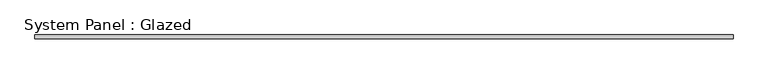
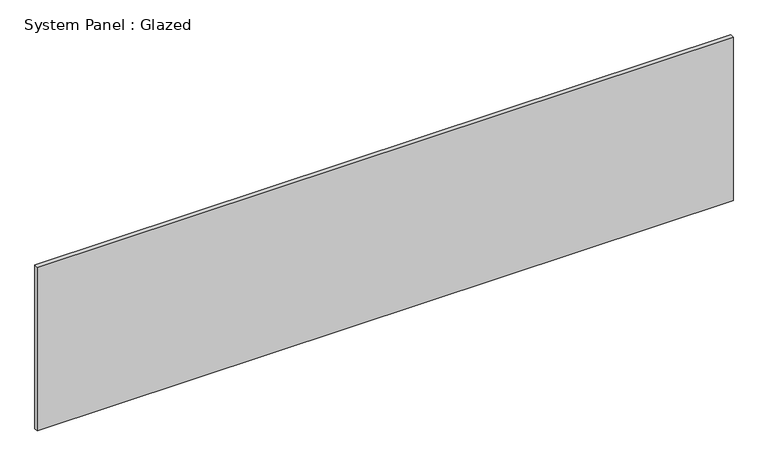
"""IFC4 building model written with IfcOpenShell, lengths in millimetres: plate geometry, System Panel : Glazed."""

from ifc_helpers import new_model, si_unit, origin, origin_with_axes, place, context, project, spatial, polyline, outline, extrude, source, transform, mapped, element, save


def system_panel_glazed_d304929f(model_context):
    return source(origin(), model_context, "Body", "SweptSolid", [
        extrude(outline(polyline([(2321.8812126, 19.05), (-2321.8812126, 19.05), (-2321.8812126, 44.45), (2321.8812126, 44.45), (2321.8812126, 19.05)])), origin_with_axes(), (0.0, 0.0, 1.0), 1155.7),
    ])


if __name__ == "__main__":
    model = new_model("IFC4")
    model_context = context("Model", 3, world=origin())
    ifc_project = project(units=[si_unit("LENGTHUNIT", "METRE", prefix="MILLI")], contexts=[model_context])
    site = spatial("IfcSite", under=ifc_project)
    building = spatial("IfcBuilding", under=site)
    placement = place(None, origin())
    system_panel_glazed_shape = system_panel_glazed_d304929f(model_context)
    element("IfcPlate", 1, ObjectType="System Panel : Glazed", at=placement, inside=building, context=model_context, shape_type="MappedRepresentation", body=[
        mapped(system_panel_glazed_shape, transform((0.0, 0.0, 0.0), x_axis=(1.0, 0.0, 0.0), y_axis=(0.0, 1.0, 0.0), z_axis=(0.0, 0.0, 1.0))),
    ])
    save(model, "model.ifc")

# Revit data of these elements
# Type "System Panel : Glazed"
#   Construction Type Id = "GSP4R"
#   Analytic Construction = "1/8 in Pilkington single glazing"
#   Visual Light Transmittance = 0.9
#   Solar Heat Gain Coefficient = 0.86
#   Heat Transfer Coefficient (U) = 1.18115 BTU/(h·ft²·°F)
# Element 1 (IfcPlate, "System Panel : Glazed")
#   Materials on its faces: "Glass"
# Materials
#   "Glass": class "Glass", colour RGB 0 128 192, transparency 0.75, Description = "Soda Lime Glass", Cost = 0
